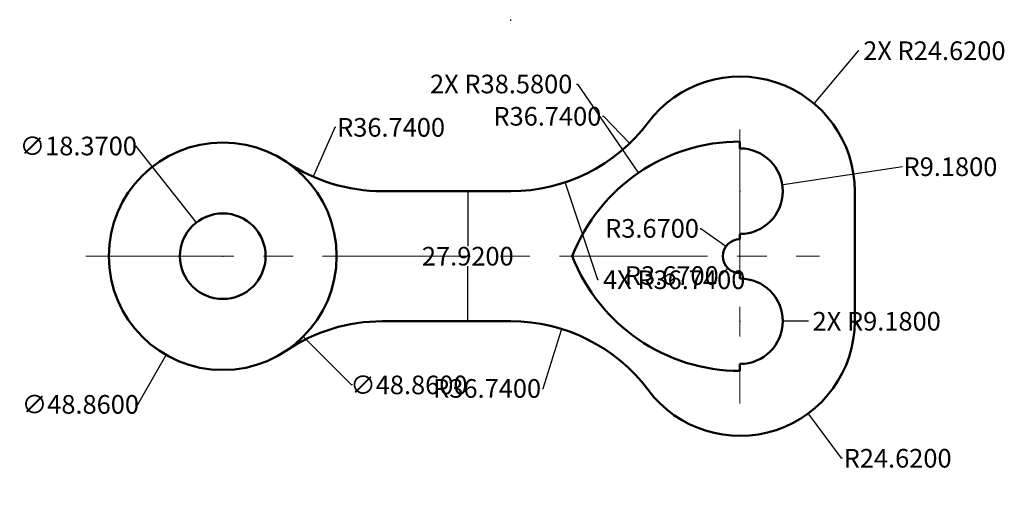
# Model space of a CAD drawing. Units: inches. Extents: x 237 to 449, y 165 to 267.
import ezdxf

# ---------------------------------------------------------------- set-up
doc = ezdxf.new("R2010")
doc.units = ezdxf.units.IN
doc.header["$MEASUREMENT"] = 0
doc.linetypes.add('CENTER', pattern=[50.8, 31.75, -6.35, 6.35, -6.35])
for name, color, linetype, lineweight in [('M-CNTR', 4, 'CENTER', 18), ('M-DIMS', 2, 'Continuous', 25), ('M-OUTL', 7, 'Continuous', 50)]:
    doc.layers.add(name, color=color, linetype=linetype, lineweight=lineweight)
doc.styles.get("Standard").update_dxf_attribs({"font": 'arial.ttf'})
doc.dimstyles.get("Standard").update_dxf_attribs({"dimtxt": 4, "dimasz": 0.18, "dimexe": 0.18, "dimexo": 0.0625, "dimgap": 0.09, "dimtad": 0, "dimtih": 1, "dimtoh": 1, "dimdec": 4, "dimzin": 0, "dimdsep": 46, "dimtxsty": 'Standard', "dimcen": 0.09, "dimadec": 0, "dimazin": 0, "dimtfac": 1, "dimtdec": 4, "dimtofl": 0, "dimtmove": 0, "dimatfit": 3, "dimfxl": 1, "dimtolj": 1, "dimtzin": 0, "dimarcsym": 0})

# ---------------------------------------------------------------- blocks, each defined once
blk = doc.blocks.new('*D1')
at = {"layer": 'Defpoints', "color": 0, "transparency": 16777216}
for p in [(315.13, 266.55), (300.31, 232.93)]:
    blk.add_point(p, dxfattribs=at)
at = {"layer": 'M-DIMS', "color": 0, "lineweight": -2, "transparency": 16777216}
for p, q in [((304.97, 243.51), (300.38, 233.09)), ((305.15, 243.51), (304.97, 243.51))]:
    blk.add_line(p, q, dxfattribs=at)
at = {"layer": 'M-DIMS', "color": 0, "transparency": 16777216}
blk.add_solid([(300.35, 233.11), (300.41, 233.08), (300.31, 232.93)], dxfattribs=at)
at = {"layer": 'M-DIMS', "color": 0, "transparency": 16777216, "insert": (317.01, 243.51), "char_height": 4, "attachment_point": 5}
blk.add_mtext('\\A1;R36.7400', dxfattribs=at)
blk = doc.blocks.new('*D2')
at = {"layer": 'Defpoints', "color": 0, "transparency": 16777216}
for p in [(353.64, 200.22), (342.71, 165.15)]:
    blk.add_point(p, dxfattribs=at)
at = {"layer": 'M-DIMS', "color": 0, "lineweight": -2, "transparency": 16777216}
for p, q in [((349.66, 187.45), (353.58, 200.05)), ((349.48, 187.45), (349.66, 187.45))]:
    blk.add_line(p, q, dxfattribs=at)
at = {"layer": 'M-DIMS', "color": 0, "transparency": 16777216}
blk.add_solid([(353.55, 200.06), (353.61, 200.04), (353.64, 200.22)], dxfattribs=at)
at = {"layer": 'M-DIMS', "color": 0, "transparency": 16777216, "insert": (337.62, 187.45), "char_height": 4, "attachment_point": 5}
blk.add_mtext('\\A1;R36.7400', dxfattribs=at)
blk = doc.blocks.new('*D3')
at = {"layer": 'Defpoints', "color": 0, "transparency": 16777216}
for p in [(391.86, 201.89), (406.51, 182.1)]:
    blk.add_point(p, dxfattribs=at)
at = {"layer": 'M-DIMS', "color": 0, "lineweight": -2, "transparency": 16777216}
for p, q in [((391.77, 201.89), (391.95, 201.89)), ((391.86, 201.8), (391.86, 201.98)), ((413.64, 172.46), (406.62, 181.95)), ((413.82, 172.46), (413.64, 172.46))]:
    blk.add_line(p, q, dxfattribs=at)
at = {"layer": 'M-DIMS', "color": 0, "transparency": 16777216}
blk.add_solid([(406.64, 181.97), (406.59, 181.94), (406.51, 182.1)], dxfattribs=at)
at = {"layer": 'M-DIMS', "color": 0, "transparency": 16777216, "insert": (425.67, 172.46), "char_height": 4, "attachment_point": 5}
blk.add_mtext('\\A1;R24.6200', dxfattribs=at)
blk = doc.blocks.new('*D4')
at = {"layer": 'Defpoints', "color": 0, "transparency": 16777216}
for p in [(400.94, 231.17), (391.86, 229.81)]:
    blk.add_point(p, dxfattribs=at)
at = {"layer": 'M-DIMS', "color": 0, "lineweight": -2, "transparency": 16777216}
for p, q in [((426.7, 235.06), (401.11, 231.2)), ((391.77, 229.81), (391.95, 229.81)), ((391.86, 229.72), (391.86, 229.9))]:
    blk.add_line(p, q, dxfattribs=at)
at = {"layer": 'M-DIMS', "color": 0, "transparency": 16777216}
blk.add_solid([(401.11, 231.23), (401.12, 231.17), (400.94, 231.17)], dxfattribs=at)
at = {"layer": 'M-DIMS', "color": 0, "transparency": 16777216, "insert": (437, 235.06), "char_height": 4, "attachment_point": 5}
blk.add_mtext('\\A1;R9.1800', dxfattribs=at)
blk = doc.blocks.new('*D5')
at = {"layer": 'Defpoints', "color": 0, "transparency": 16777216}
for p in [(342.71, 266.55), (368.17, 240.06)]:
    blk.add_point(p, dxfattribs=at)
at = {"layer": 'M-DIMS', "color": 0, "lineweight": -2, "transparency": 16777216}
for p, q in [((362.39, 245.89), (362.57, 245.89)), ((362.57, 245.89), (368.05, 240.19))]:
    blk.add_line(p, q, dxfattribs=at)
at = {"layer": 'M-DIMS', "color": 0, "transparency": 16777216}
blk.add_solid([(368.07, 240.21), (368.03, 240.17), (368.17, 240.06)], dxfattribs=at)
at = {"layer": 'M-DIMS', "color": 0, "transparency": 16777216, "insert": (350.54, 245.89), "char_height": 4, "attachment_point": 5}
blk.add_mtext('\\A1;R36.7400', dxfattribs=at)
blk = doc.blocks.new('*D6')
at = {"layer": 'Defpoints', "color": 0, "transparency": 16777216}
for p in [(275.22, 223.05), (286.6, 208.64)]:
    blk.add_point(p, dxfattribs=at)
at = {"layer": 'M-DIMS', "color": 0, "lineweight": -2, "transparency": 16777216}
for p, q in [((262.04, 239.51), (262.22, 239.51)), ((262.22, 239.51), (275.1, 223.19)), ((280.82, 215.85), (281, 215.85)), ((280.91, 215.76), (280.91, 215.94))]:
    blk.add_line(p, q, dxfattribs=at)
at = {"layer": 'M-DIMS', "color": 0, "transparency": 16777216}
blk.add_solid([(275.13, 223.21), (275.08, 223.18), (275.22, 223.05)], dxfattribs=at)
at = {"layer": 'M-DIMS', "color": 0, "transparency": 16777216, "insert": (249.93, 239.51), "char_height": 4, "attachment_point": 5}
blk.add_mtext('\\A1;∅18.3700', dxfattribs=at)
blk = doc.blocks.new('*D7')
at = {"layer": 'Defpoints', "color": 0, "transparency": 16777216}
for p in [(293.06, 237.04), (268.76, 194.65)]:
    blk.add_point(p, dxfattribs=at)
at = {"layer": 'M-DIMS', "color": 0, "lineweight": -2, "transparency": 16777216}
for p, q in [((280.82, 215.85), (281, 215.85)), ((280.91, 215.76), (280.91, 215.94)), ((262.67, 184.03), (268.67, 194.5)), ((262.49, 184.03), (262.67, 184.03))]:
    blk.add_line(p, q, dxfattribs=at)
at = {"layer": 'M-DIMS', "color": 0, "transparency": 16777216}
blk.add_solid([(268.64, 194.51), (268.69, 194.48), (268.76, 194.65)], dxfattribs=at)
at = {"layer": 'M-DIMS', "color": 0, "transparency": 16777216, "insert": (250.37, 184.03), "char_height": 4, "attachment_point": 5}
blk.add_mtext('\\A1;∅48.8600', dxfattribs=at)
blk = doc.blocks.new('*D8')
at = {"layer": 'Defpoints', "color": 0, "transparency": 16777216}
for p in [(328.92, 229.81), (328.92, 201.89), (333.47, 201.89)]:
    blk.add_point(p, dxfattribs=at)
at = {"layer": 'M-DIMS', "color": 0, "lineweight": -2, "transparency": 16777216}
for p, q in [((328.99, 229.81), (333.65, 229.81)), ((333.47, 229.63), (333.47, 217.98)), ((333.47, 202.07), (333.47, 213.71)), ((328.99, 201.89), (333.65, 201.89))]:
    blk.add_line(p, q, dxfattribs=at)
at = {"layer": 'M-DIMS', "color": 0, "transparency": 16777216}
for points in [[(333.44, 229.63), (333.5, 229.63), (333.47, 229.81)], [(333.44, 202.07), (333.5, 202.07), (333.47, 201.89)]]:
    blk.add_solid(points, dxfattribs=at)
at = {"layer": 'M-DIMS', "color": 0, "transparency": 16777216, "insert": (333.47, 215.85), "char_height": 4, "attachment_point": 5}
blk.add_mtext('\\A1;27.9200', dxfattribs=at)
blk = doc.blocks.new('*D9')
at = {"layer": 'Defpoints', "color": 0, "transparency": 16777216}
for p in [(388.87, 217.98), (391.86, 215.85)]:
    blk.add_point(p, dxfattribs=at)
at = {"layer": 'M-DIMS', "color": 0, "lineweight": -2, "transparency": 16777216}
for p, q in [((383.3, 221.82), (383.48, 221.82)), ((383.48, 221.82), (388.72, 218.08)), ((391.77, 215.85), (391.95, 215.85)), ((391.86, 215.76), (391.86, 215.94))]:
    blk.add_line(p, q, dxfattribs=at)
at = {"layer": 'M-DIMS', "color": 0, "transparency": 16777216}
blk.add_solid([(388.74, 218.1), (388.71, 218.06), (388.87, 217.98)], dxfattribs=at)
at = {"layer": 'M-DIMS', "color": 0, "transparency": 16777216, "insert": (372.99, 221.82), "char_height": 4, "attachment_point": 5}
blk.add_mtext('\\A1;R3.6700', dxfattribs=at)
blk = doc.blocks.new('*D10')
at = {"layer": 'Defpoints', "color": 0, "transparency": 16777216}
for p in [(263.63, 233.12), (298.18, 198.57)]:
    blk.add_point(p, dxfattribs=at)
at = {"layer": 'M-DIMS', "color": 0, "lineweight": -2, "transparency": 16777216}
for p, q in [((280.82, 215.85), (281, 215.85)), ((280.91, 215.76), (280.91, 215.94)), ((308.55, 188.21), (298.31, 198.44)), ((308.73, 188.21), (308.55, 188.21))]:
    blk.add_line(p, q, dxfattribs=at)
at = {"layer": 'M-DIMS', "color": 0, "transparency": 16777216}
blk.add_solid([(298.33, 198.46), (298.29, 198.42), (298.18, 198.57)], dxfattribs=at)
at = {"layer": 'M-DIMS', "color": 0, "transparency": 16777216, "insert": (320.84, 188.21), "char_height": 4, "attachment_point": 5}
blk.add_mtext('\\A1;∅48.8600', dxfattribs=at)
blk = doc.blocks.new('*D11')
at = {"layer": 'Defpoints', "color": 0, "transparency": 16777216}
for p in [(370.07, 233.72), (391.86, 201.89)]:
    blk.add_point(p, dxfattribs=at)
at = {"layer": 'M-DIMS', "color": 0, "lineweight": -2, "transparency": 16777216}
for p, q in [((356.81, 252.82), (356.99, 252.82)), ((356.99, 252.82), (369.96, 233.87)), ((391.77, 201.89), (391.95, 201.89)), ((391.86, 201.8), (391.86, 201.98))]:
    blk.add_line(p, q, dxfattribs=at)
at = {"layer": 'M-DIMS', "color": 0, "transparency": 16777216}
blk.add_solid([(369.99, 233.89), (369.94, 233.85), (370.07, 233.72)], dxfattribs=at)
at = {"layer": 'M-DIMS', "color": 0, "transparency": 16777216, "insert": (340.63, 252.82), "char_height": 4, "attachment_point": 5}
blk.add_mtext('\\A1;2X R38.5800', dxfattribs=at)
blk = doc.blocks.new('*D12')
at = {"layer": 'Defpoints', "color": 0, "transparency": 16777216}
for p in [(407.69, 248.66), (391.86, 229.81)]:
    blk.add_point(p, dxfattribs=at)
at = {"layer": 'M-DIMS', "color": 0, "lineweight": -2, "transparency": 16777216}
for p, q in [((417.19, 259.97), (407.81, 248.8)), ((417.37, 259.97), (417.19, 259.97)), ((391.77, 229.81), (391.95, 229.81)), ((391.86, 229.72), (391.86, 229.9))]:
    blk.add_line(p, q, dxfattribs=at)
at = {"layer": 'M-DIMS', "color": 0, "transparency": 16777216}
blk.add_solid([(407.78, 248.82), (407.83, 248.78), (407.69, 248.66)], dxfattribs=at)
at = {"layer": 'M-DIMS', "color": 0, "transparency": 16777216, "insert": (433.55, 259.97), "char_height": 4, "attachment_point": 5}
blk.add_mtext('\\A1;2X R24.6200', dxfattribs=at)
blk = doc.blocks.new('*D13')
at = {"layer": 'Defpoints', "color": 0, "transparency": 16777216}
for p in [(391.86, 201.89), (401.04, 201.88)]:
    blk.add_point(p, dxfattribs=at)
at = {"layer": 'M-DIMS', "color": 0, "lineweight": -2, "transparency": 16777216}
for p, q in [((391.77, 201.89), (391.95, 201.89)), ((391.86, 201.8), (391.86, 201.98)), ((406.55, 201.88), (401.22, 201.88))]:
    blk.add_line(p, q, dxfattribs=at)
at = {"layer": 'M-DIMS', "color": 0, "transparency": 16777216}
blk.add_solid([(401.22, 201.91), (401.22, 201.85), (401.04, 201.88)], dxfattribs=at)
at = {"layer": 'M-DIMS', "color": 0, "transparency": 16777216, "insert": (421.18, 201.88), "char_height": 4, "attachment_point": 5}
blk.add_mtext('\\A1;2X R9.1800', dxfattribs=at)
blk = doc.blocks.new('*D14')
at = {"layer": 'Defpoints', "color": 0, "transparency": 16777216}
for p in [(391.86, 215.85), (389.26, 213.25)]:
    blk.add_point(p, dxfattribs=at)
at = {"layer": 'M-DIMS', "color": 0, "lineweight": -2, "transparency": 16777216}
for p, q in [((391.77, 215.85), (391.95, 215.85)), ((391.86, 215.76), (391.86, 215.94)), ((387.53, 211.69), (387.71, 211.69)), ((387.71, 211.69), (389.14, 213.12))]:
    blk.add_line(p, q, dxfattribs=at)
at = {"layer": 'M-DIMS', "color": 0, "transparency": 16777216}
blk.add_solid([(389.12, 213.14), (389.16, 213.1), (389.26, 213.25)], dxfattribs=at)
at = {"layer": 'M-DIMS', "color": 0, "transparency": 16777216, "insert": (377.23, 211.69), "char_height": 4, "attachment_point": 5}
blk.add_mtext('\\A1;R3.6700', dxfattribs=at)
blk = doc.blocks.new('*D15')
at = {"layer": 'Defpoints', "color": 0, "transparency": 16777216}
for p in [(342.71, 266.55), (354.35, 231.7)]:
    blk.add_point(p, dxfattribs=at)
at = {"layer": 'M-DIMS', "color": 0, "lineweight": -2, "transparency": 16777216}
for p, q in [((342.62, 266.55), (342.8, 266.55)), ((342.71, 266.46), (342.71, 266.64)), ((361.33, 210.79), (354.41, 231.53)), ((361.51, 210.79), (361.33, 210.79))]:
    blk.add_line(p, q, dxfattribs=at)
at = {"layer": 'M-DIMS', "color": 0, "transparency": 16777216}
blk.add_solid([(354.43, 231.53), (354.38, 231.52), (354.35, 231.7)], dxfattribs=at)
at = {"layer": 'M-DIMS', "color": 0, "transparency": 16777216, "insert": (377.74, 210.79), "char_height": 4, "attachment_point": 5}
blk.add_mtext('\\A1;4X R36.7400', dxfattribs=at)

msp = doc.modelspace()

# ---------------------------------------------------------------- linework, layer by layer
at = {"layer": 'M-CNTR'}
for p, q in [((391.85874, 243.04704), (391.85874, 184.25192)), ((251.53268, 215.84513), (408.88933, 215.84513))]:
    msp.add_line(p, q, dxfattribs=at)
at = {"layer": 'M-OUTL'}
for p, q in [((391.85874, 238.98513), (391.85874, 240.46513)), ((342.71383, 229.80513), (315.13269, 229.80513)), ((416.47874, 201.88513), (416.47874, 229.80513)), ((391.85874, 219.51513), (391.85874, 220.62513)), ((391.85874, 220.62513), (391.85874, 219.51513)), ((391.85874, 212.17513), (391.85874, 211.06513)), ((391.85874, 212.17513), (391.85874, 211.06513)), ((342.71383, 201.88513), (315.13269, 201.88513)), ((391.85874, 192.70513), (391.85874, 191.22513))]:
    msp.add_line(p, q, dxfattribs=at)
for radius in [24.43, 9.185]:
    msp.add_circle((280.90874, 215.84513), radius, dxfattribs=at)
for centre, radius, start, end in [((391.85874, 229.80513), 24.62, 0, 143.2187586), ((342.71383, 266.54513), 36.74, 270, 323.2187586), ((391.85874, 201.88513), 38.58, 90, 158.7864212), ((391.85874, 229.80513), 9.18, 270, 90), ((315.13269, 266.54513), 36.74, 235.9795226, 270), ((391.85874, 215.84513), 3.67, 90, 270), ((391.85874, 229.80513), 38.58, 201.2135788, 270), ((391.85874, 201.88513), 9.18, 270, 90), ((315.13269, 165.14513), 36.74, 90, 124.0204774), ((342.71383, 165.14513), 36.74, 36.7812414, 90), ((391.85874, 201.88513), 24.62, 216.7812414, 0)]:
    msp.add_arc(centre, radius, start, end, dxfattribs=at)

# ---------------------------------------------------------------- dimensions: what is measured, and where the dimension line sits
at = {"layer": 'M-DIMS'}
for center, mpoint, override, picture, middle in [((315.13269, 266.54513), (300.30694, 232.92928), {"dimclrd": 0, "dimclre": 0, "dimclrt": 0}, '*D1', (317.00855, 243.51263)), ((342.71383, 266.54513), (368.17498, 240.0582), {"dimclrd": 0, "dimclre": 0, "dimclrt": 0}, '*D5', (350.53905, 245.88583)), ((391.85874, 229.80513), (400.93617, 231.17358), {"dimclrd": 0, "dimclre": 0, "dimclrt": 0}, '*D4', (426.70329, 235.05809)), ((391.85874, 215.84513), (388.87017, 217.97524), {"dimclrd": 0, "dimclre": 0, "dimclrt": 0}, '*D9', (372.995, 221.82061)), ((391.85874, 215.84512), (389.26385, 213.24985), {"dimdec": 4, "dimlfac": 1, "dimrnd": 0, "dimzin": 0, "dimdsep": 46, "dimlunit": 2}, '*D14', (377.22682, 211.69268)), ((391.85874, 201.88513), (406.50809, 182.09774), {"dimclrd": 0, "dimclre": 0, "dimclrt": 0}, '*D3', (425.6737, 172.4648)), ((342.71383, 165.14513), (353.63686, 200.22382), {"dimclrd": 0, "dimclre": 0, "dimclrt": 0}, '*D2', (337.62393, 187.44566))]:
    dim = msp.add_radius_dim(center=center, mpoint=mpoint, dimstyle='Standard', override=override, dxfattribs=at)
    dim.commit()
    dim.dimension.update_dxf_attribs({"geometry": picture, "text_midpoint": middle, "dimtype": 164})
for center, mpoint, text, picture, middle in [((342.71383, 266.54512), (354.3482, 231.69589), '4X <>', '*D15', (377.74071, 210.78635)), ((391.85874, 229.80513), (407.69024, 248.66005), '2X <>', '*D12', (433.55463, 259.973)), ((391.85874, 201.88512), (370.06622, 233.72068), '2X <>', '*D11', (340.62521, 252.82201)), ((391.85874, 201.88512), (401.03874, 201.885), '2X <>', '*D13', (406.54674, 201.88493))]:
    dim = msp.add_radius_dim(center=center, mpoint=mpoint, text=text, dimstyle='Standard', override={"dimdec": 4, "dimlfac": 1, "dimrnd": 0, "dimzin": 0, "dimdsep": 46, "dimlunit": 2}, dxfattribs=at)
    dim.commit()
    dim.dimension.update_dxf_attribs({"geometry": picture, "text_midpoint": middle, "dimtype": 164})
for p1, p2, override, picture, middle in [((286.60141, 208.63695), (275.21607, 223.0533), {"dimclrd": 0, "dimclre": 0, "dimclrt": 0}, '*D6', (249.92514, 239.50785)), ((293.06186, 237.03773), (268.75561, 194.65252), {"dimclrd": 0, "dimclre": 0, "dimclrt": 0}, '*D7', (250.37048, 184.03418)), ((263.63405, 233.11968), (298.18342, 198.57057), {"dimdec": 4, "dimlfac": 1, "dimrnd": 0, "dimzin": 0, "dimdsep": 46, "dimlunit": 2}, '*D10', (320.84416, 188.20585))]:
    dim = msp.add_diameter_dim_2p(p1=p1, p2=p2, dimstyle='Standard', override=override, dxfattribs=at)
    dim.commit()
    dim.dimension.update_dxf_attribs({"geometry": picture, "text_midpoint": middle, "dimtype": 163})
dim = msp.add_linear_dim(base=(333.47227, 201.88513), p1=(328.92326, 229.80513), p2=(328.92326, 201.88513), angle=90, dimstyle='Standard', override={"dimclrd": 0, "dimclre": 0, "dimclrt": 0}, dxfattribs=at)
dim.commit()
dim.dimension.update_dxf_attribs({"geometry": '*D8', "text_midpoint": (333.47227, 215.84513)})

doc.saveas('drawing.dxf')
